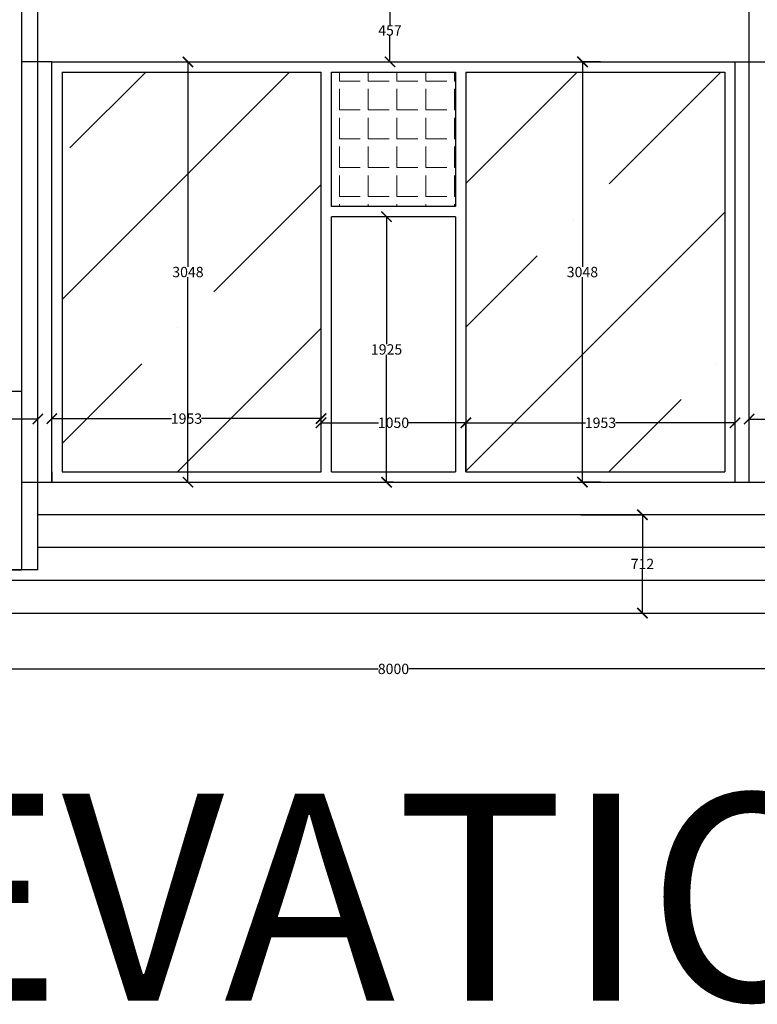
# Model space of a CAD drawing. Units: inches. Extents: x 829 to 33356404, y 1874 to 16983.
# Tile 6 of 9: x 10848 to 16199, y 1874 to 9014. Entities that reach past the tile are written whole.
import ezdxf

# ---------------------------------------------------------------- set-up
doc = ezdxf.new("R2010")
doc.units = ezdxf.units.IN
doc.header["$MEASUREMENT"] = 0
doc.header["$PDMODE"] = 3
for name, color, linetype, lineweight in [('A-ANNO-DIMS', 2, 'Continuous', 18), ('A-ANNO-TEXT', 7, 'Continuous', 25), ('A-ELEV', 7, 'Continuous', 25), ('A-ELEV-PATT', 8, 'Continuous', 13)]:
    doc.layers.add(name, color=color, linetype=linetype, lineweight=lineweight)
doc.styles.get("Standard").update_dxf_attribs({"font": 'arial.ttf'})
doc.dimstyles.get("Standard").update_dxf_attribs({"dimtxt": 75, "dimasz": 75, "dimexe": 0.18, "dimexo": 0.0625, "dimgap": 0.09, "dimtad": 0, "dimtih": 1, "dimtoh": 1, "dimdec": 0, "dimzin": 0, "dimdsep": 46, "dimtxsty": 'Standard', "dimblk": 'ARCHTICK', "dimcen": 0.09, "dimadec": 0, "dimazin": 0, "dimtfac": 1, "dimtdec": 0, "dimtofl": 0, "dimtmove": 0, "dimatfit": 3, "dimfxl": 1, "dimtolj": 1, "dimtzin": 0, "dimarcsym": 0})

# ---------------------------------------------------------------- blocks, each defined once
blk = doc.blocks.new('_ArchTick')
at = {"color": 0, "linetype": 'ByBlock', "const_width": 0.15}
blk.add_lwpolyline([(-0.5, -0.5), (0.5, 0.5)], dxfattribs=at)
blk = doc.blocks.new('*D3')
at = {"layer": 'A-ANNO-DIMS', "color": 0, "lineweight": -2, "transparency": 16777216}
for p, q in [((9559.8, 4746.4), (9559.8, 4306.1)), ((17559.8, 4746.4), (17559.8, 4306.1)), ((9559.8, 4306.3), (13447.8, 4306.3)), ((17559.8, 4306.3), (13671.8, 4306.3))]:
    blk.add_line(p, q, dxfattribs=at)
at = {"layer": 'Defpoints', "color": 0, "transparency": 16777216}
for p in [(9559.8, 4746.5), (17559.8, 4746.5), (17559.8, 4306.3)]:
    blk.add_point(p, dxfattribs=at)
at = {"layer": 'A-ANNO-DIMS', "color": 0, "lineweight": -2, "transparency": 16777216, "xscale": 75, "yscale": 75, "zscale": 75, "rotation": 180}
blk.add_blockref('_ArchTick', (9559.8, 4306.3), dxfattribs=at)
at = {"layer": 'A-ANNO-DIMS', "color": 0, "lineweight": -2, "transparency": 16777216, "xscale": 75, "yscale": 75, "zscale": 75}
blk.add_blockref('_ArchTick', (17559.8, 4306.3), dxfattribs=at)
at = {"layer": 'A-ANNO-DIMS', "color": 0, "transparency": 16777216, "insert": (13559.8, 4306.3), "char_height": 75, "attachment_point": 5}
blk.add_mtext('\\A1;8000', dxfattribs=at)
blk = doc.blocks.new('*D17')
at = {"layer": 'A-ANNO-DIMS', "color": 0, "lineweight": -2, "transparency": 16777216}
for p, q in [((9559.8, 5735.5), (9559.8, 6118.2)), ((9559.8, 6118), (10161.4, 6118)), ((10979.9, 6118), (10378.3, 6118)), ((10979.9, 5735.5), (10979.9, 6118.2))]:
    blk.add_line(p, q, dxfattribs=at)
at = {"layer": 'Defpoints', "color": 0, "transparency": 16777216}
for p in [(9559.8, 6118), (9559.8, 5735.5), (10979.9, 5735.5)]:
    blk.add_point(p, dxfattribs=at)
at = {"layer": 'A-ANNO-DIMS', "color": 0, "lineweight": -2, "transparency": 16777216, "xscale": 75, "yscale": 75, "zscale": 75, "rotation": 180}
blk.add_blockref('_ArchTick', (9559.8, 6118), dxfattribs=at)
at = {"layer": 'A-ANNO-DIMS', "color": 0, "lineweight": -2, "transparency": 16777216, "xscale": 75, "yscale": 75, "zscale": 75}
blk.add_blockref('_ArchTick', (10979.9, 6118), dxfattribs=at)
at = {"layer": 'A-ANNO-DIMS', "color": 0, "transparency": 16777216, "insert": (10269.9, 6118), "char_height": 75, "attachment_point": 5}
blk.add_mtext('\\A1;1420', dxfattribs=at)
blk = doc.blocks.new('*D18')
at = {"layer": 'A-ANNO-DIMS', "color": 0, "lineweight": -2, "transparency": 16777216}
for p, q in [((16139.7, 5735.5), (16139.7, 6118.2)), ((16139.7, 6118), (16741.3, 6118)), ((17559.8, 6118), (16958.2, 6118)), ((17559.8, 5735.5), (17559.8, 6118.2))]:
    blk.add_line(p, q, dxfattribs=at)
at = {"layer": 'Defpoints', "color": 0, "transparency": 16777216}
for p in [(16139.7, 6118), (16139.7, 5735.5), (17559.8, 5735.5)]:
    blk.add_point(p, dxfattribs=at)
at = {"layer": 'A-ANNO-DIMS', "color": 0, "lineweight": -2, "transparency": 16777216, "xscale": 75, "yscale": 75, "zscale": 75, "rotation": 180}
blk.add_blockref('_ArchTick', (16139.7, 6118), dxfattribs=at)
at = {"layer": 'A-ANNO-DIMS', "color": 0, "lineweight": -2, "transparency": 16777216, "xscale": 75, "yscale": 75, "zscale": 75}
blk.add_blockref('_ArchTick', (17559.8, 6118), dxfattribs=at)
at = {"layer": 'A-ANNO-DIMS', "color": 0, "transparency": 16777216, "insert": (16849.7, 6118), "char_height": 75, "attachment_point": 5}
blk.add_mtext('\\A1;1420', dxfattribs=at)
blk = doc.blocks.new('*D19')
at = {"layer": 'A-ANNO-DIMS', "color": 0, "lineweight": -2, "transparency": 16777216}
for p, q in [((14084.8, 5735.5), (14084.8, 6091.3)), ((14084.8, 6091.1), (14952.7, 6091.1)), ((16037.8, 6091.1), (15169.8, 6091.1)), ((16037.8, 5735.5), (16037.8, 6091.3))]:
    blk.add_line(p, q, dxfattribs=at)
at = {"layer": 'Defpoints', "color": 0, "transparency": 16777216}
for p in [(16037.8, 6091.1), (14084.8, 5735.5), (16037.8, 5735.5)]:
    blk.add_point(p, dxfattribs=at)
at = {"layer": 'A-ANNO-DIMS', "color": 0, "lineweight": -2, "transparency": 16777216, "xscale": 75, "yscale": 75, "zscale": 75, "rotation": 180}
blk.add_blockref('_ArchTick', (14084.8, 6091.1), dxfattribs=at)
at = {"layer": 'A-ANNO-DIMS', "color": 0, "lineweight": -2, "transparency": 16777216, "xscale": 75, "yscale": 75, "zscale": 75}
blk.add_blockref('_ArchTick', (16037.8, 6091.1), dxfattribs=at)
at = {"layer": 'A-ANNO-DIMS', "color": 0, "transparency": 16777216, "insert": (15061.3, 6091.1), "char_height": 75, "attachment_point": 5}
blk.add_mtext('\\A1;1953', dxfattribs=at)
blk = doc.blocks.new('*D20')
at = {"layer": 'A-ANNO-DIMS', "color": 0, "lineweight": -2, "transparency": 16777216}
for p, q in [((11081.8, 5735.5), (11081.8, 6121.5)), ((11081.8, 6121.3), (11949.7, 6121.3)), ((13034.8, 6121.3), (12166.8, 6121.3)), ((13034.8, 5735.5), (13034.8, 6121.5))]:
    blk.add_line(p, q, dxfattribs=at)
at = {"layer": 'Defpoints', "color": 0, "transparency": 16777216}
for p in [(13034.8, 6121.3), (11081.8, 5735.5), (13034.8, 5735.5)]:
    blk.add_point(p, dxfattribs=at)
at = {"layer": 'A-ANNO-DIMS', "color": 0, "lineweight": -2, "transparency": 16777216, "xscale": 75, "yscale": 75, "zscale": 75, "rotation": 180}
blk.add_blockref('_ArchTick', (11081.8, 6121.3), dxfattribs=at)
at = {"layer": 'A-ANNO-DIMS', "color": 0, "lineweight": -2, "transparency": 16777216, "xscale": 75, "yscale": 75, "zscale": 75}
blk.add_blockref('_ArchTick', (13034.8, 6121.3), dxfattribs=at)
at = {"layer": 'A-ANNO-DIMS', "color": 0, "transparency": 16777216, "insert": (12058.3, 6121.3), "char_height": 75, "attachment_point": 5}
blk.add_mtext('\\A1;1953', dxfattribs=at)
blk = doc.blocks.new('*D21')
at = {"layer": 'A-ANNO-DIMS', "color": 0, "lineweight": -2, "transparency": 16777216}
for p, q in [((15061.2, 8708.5), (14930.7, 8708.5)), ((14930.8, 8708.5), (14930.8, 7222.9)), ((14930.8, 5660.5), (14930.8, 7146.1)), ((15061.2, 5660.5), (14930.7, 5660.5))]:
    blk.add_line(p, q, dxfattribs=at)
at = {"layer": 'Defpoints', "color": 0, "transparency": 16777216}
for p in [(15061.3, 8708.5), (14930.8, 5660.5), (15061.3, 5660.5)]:
    blk.add_point(p, dxfattribs=at)
at = {"layer": 'A-ANNO-DIMS', "color": 0, "lineweight": -2, "transparency": 16777216, "xscale": 75, "yscale": 75, "zscale": 75}
for p, rotation in [((14930.8, 8708.5), 90), ((14930.8, 5660.5), 270)]:
    blk.add_blockref('_ArchTick', p, dxfattribs=dict(at, rotation=rotation))
at = {"layer": 'A-ANNO-DIMS', "color": 0, "transparency": 16777216, "insert": (14930.8, 7184.5), "char_height": 75, "attachment_point": 5}
blk.add_mtext('\\A1;3048', dxfattribs=at)
blk = doc.blocks.new('*D24')
at = {"layer": 'A-ANNO-DIMS', "color": 0, "lineweight": -2, "transparency": 16777216}
for p, q in [((13534.6, 9165.5), (13534.3, 9165.5)), ((13534.5, 9165.5), (13534.5, 8975.2)), ((13534.5, 8708.5), (13534.5, 8898.7)), ((13534.6, 8708.5), (13534.3, 8708.5))]:
    blk.add_line(p, q, dxfattribs=at)
at = {"layer": 'Defpoints', "color": 0, "transparency": 16777216}
for p in [(13534.7, 9165.5), (13534.5, 8708.5), (13534.7, 8708.5)]:
    blk.add_point(p, dxfattribs=at)
at = {"layer": 'A-ANNO-DIMS', "color": 0, "lineweight": -2, "transparency": 16777216, "xscale": 75, "yscale": 75, "zscale": 75}
for p, rotation in [((13534.5, 9165.5), 90), ((13534.5, 8708.5), 270)]:
    blk.add_blockref('_ArchTick', p, dxfattribs=dict(at, rotation=rotation))
at = {"layer": 'A-ANNO-DIMS', "color": 0, "transparency": 16777216, "insert": (13534.5, 8937), "char_height": 75, "attachment_point": 5}
blk.add_mtext('\\A1;457', dxfattribs=at)
blk = doc.blocks.new('*D34')
at = {"layer": 'A-ANNO-DIMS', "color": 0, "lineweight": -2, "transparency": 16777216}
for p, q in [((9559.8, 5735.5), (9559.8, 6118.2)), ((9559.8, 6118), (10161.4, 6118)), ((10979.9, 6118), (10378.2, 6118)), ((10979.9, 5735.5), (10979.9, 6118.2))]:
    blk.add_line(p, q, dxfattribs=at)
at = {"layer": 'Defpoints', "color": 0, "transparency": 16777216}
for p in [(10979.9, 6118), (9559.8, 5735.5), (10979.9, 5735.5)]:
    blk.add_point(p, dxfattribs=at)
at = {"layer": 'A-ANNO-DIMS', "color": 0, "lineweight": -2, "transparency": 16777216, "xscale": 75, "yscale": 75, "zscale": 75, "rotation": 180}
blk.add_blockref('_ArchTick', (9559.8, 6118), dxfattribs=at)
at = {"layer": 'A-ANNO-DIMS', "color": 0, "lineweight": -2, "transparency": 16777216, "xscale": 75, "yscale": 75, "zscale": 75}
blk.add_blockref('_ArchTick', (10979.9, 6118), dxfattribs=at)
at = {"layer": 'A-ANNO-DIMS', "color": 0, "transparency": 16777216, "insert": (10269.8, 6118), "char_height": 75, "attachment_point": 5}
blk.add_mtext('\\A1;1420', dxfattribs=at)
blk = doc.blocks.new('*D60')
at = {"layer": 'A-ANNO-DIMS', "color": 0, "lineweight": -2, "transparency": 16777216}
for p, q in [((14918.4, 5423.5), (15365.9, 5423.5)), ((15365.7, 5423.5), (15365.7, 5105.2)), ((15365.7, 4711.5), (15365.7, 5029.8)), ((14972.8, 4711.5), (15365.9, 4711.5))]:
    blk.add_line(p, q, dxfattribs=at)
at = {"layer": 'Defpoints', "color": 0, "transparency": 16777216}
for p in [(14918.4, 5423.5), (14972.7, 4711.5), (15365.7, 4711.5)]:
    blk.add_point(p, dxfattribs=at)
at = {"layer": 'A-ANNO-DIMS', "color": 0, "lineweight": -2, "transparency": 16777216, "xscale": 75, "yscale": 75, "zscale": 75}
for p, rotation in [((15365.7, 5423.5), 90), ((15365.7, 4711.5), 270)]:
    blk.add_blockref('_ArchTick', p, dxfattribs=dict(at, rotation=rotation))
at = {"layer": 'A-ANNO-DIMS', "color": 0, "transparency": 16777216, "insert": (15365.7, 5067.5), "char_height": 75, "attachment_point": 5}
blk.add_mtext('\\A1;712', dxfattribs=at)
blk = doc.blocks.new('*D61')
at = {"layer": 'A-ANNO-DIMS', "color": 0, "lineweight": -2, "transparency": 16777216}
for p, q in [((12058.3, 8708.5), (12069.1, 8708.5)), ((12068.9, 8708.5), (12068.9, 7222.9)), ((12068.9, 5660.5), (12068.9, 7146.1)), ((12058.3, 5660.5), (12069.1, 5660.5))]:
    blk.add_line(p, q, dxfattribs=at)
at = {"layer": 'Defpoints', "color": 0, "transparency": 16777216}
for p in [(12058.3, 8708.5), (12058.3, 5660.5), (12068.9, 5660.5)]:
    blk.add_point(p, dxfattribs=at)
at = {"layer": 'A-ANNO-DIMS', "color": 0, "lineweight": -2, "transparency": 16777216, "xscale": 75, "yscale": 75, "zscale": 75}
for p, rotation in [((12068.9, 8708.5), 90), ((12068.9, 5660.5), 270)]:
    blk.add_blockref('_ArchTick', p, dxfattribs=dict(at, rotation=rotation))
at = {"layer": 'A-ANNO-DIMS', "color": 0, "transparency": 16777216, "insert": (12068.9, 7184.5), "char_height": 75, "attachment_point": 5}
blk.add_mtext('\\A1;3048', dxfattribs=at)
blk = doc.blocks.new('*D62')
at = {"layer": 'A-ANNO-DIMS', "color": 0, "lineweight": -2, "transparency": 16777216}
for p, q in [((13559.7, 7585.5), (13509.7, 7585.5)), ((13509.8, 7585.5), (13509.8, 6661.4)), ((13509.8, 5660.5), (13509.8, 6584.6)), ((13559.7, 5660.5), (13509.7, 5660.5))]:
    blk.add_line(p, q, dxfattribs=at)
at = {"layer": 'Defpoints', "color": 0, "transparency": 16777216}
for p in [(13509.8, 7585.5), (13559.8, 7585.5), (13559.8, 5660.5)]:
    blk.add_point(p, dxfattribs=at)
at = {"layer": 'A-ANNO-DIMS', "color": 0, "lineweight": -2, "transparency": 16777216, "xscale": 75, "yscale": 75, "zscale": 75}
for p, rotation in [((13509.8, 7585.5), 90), ((13509.8, 5660.5), 270)]:
    blk.add_blockref('_ArchTick', p, dxfattribs=dict(at, rotation=rotation))
at = {"layer": 'A-ANNO-DIMS', "color": 0, "transparency": 16777216, "insert": (13509.8, 6623), "char_height": 75, "attachment_point": 5}
blk.add_mtext('\\A1;1925', dxfattribs=at)
blk = doc.blocks.new('*D63')
at = {"layer": 'A-ANNO-DIMS', "color": 0, "lineweight": -2, "transparency": 16777216}
for p, q in [((13034.8, 5735.5), (13034.8, 6091.4)), ((13034.8, 6091.3), (13451.4, 6091.3)), ((14084.8, 6091.3), (13668.2, 6091.3)), ((14084.8, 6091.3), (14084.8, 6091.4))]:
    blk.add_line(p, q, dxfattribs=at)
at = {"layer": 'Defpoints', "color": 0, "transparency": 16777216}
for p in [(14084.8, 6091.3), (14084.8, 6091.3), (13034.8, 5735.5)]:
    blk.add_point(p, dxfattribs=at)
at = {"layer": 'A-ANNO-DIMS', "color": 0, "lineweight": -2, "transparency": 16777216, "xscale": 75, "yscale": 75, "zscale": 75, "rotation": 180}
blk.add_blockref('_ArchTick', (13034.8, 6091.3), dxfattribs=at)
at = {"layer": 'A-ANNO-DIMS', "color": 0, "lineweight": -2, "transparency": 16777216, "xscale": 75, "yscale": 75, "zscale": 75}
blk.add_blockref('_ArchTick', (14084.8, 6091.3), dxfattribs=at)
at = {"layer": 'A-ANNO-DIMS', "color": 0, "transparency": 16777216, "insert": (13559.8, 6091.3), "char_height": 75, "attachment_point": 5}
blk.add_mtext('\\A1;1050', dxfattribs=at)
blk = doc.blocks.new('*D83')
at = {"layer": 'A-ANNO-DIMS', "color": 0, "lineweight": -2, "transparency": 16777216}
for p, q in [((13604.5, 15734.9), (985.4, 15734.9)), ((985.6, 15734.9), (985.6, 10279.1)), ((985.6, 4746.5), (985.6, 10202.3)), ((3169.7, 4746.5), (985.4, 4746.5))]:
    blk.add_line(p, q, dxfattribs=at)
at = {"layer": 'Defpoints', "color": 0, "transparency": 16777216}
for p in [(985.6, 15734.9), (13604.5, 15734.9), (3169.8, 4746.5)]:
    blk.add_point(p, dxfattribs=at)
at = {"layer": 'A-ANNO-DIMS', "color": 0, "lineweight": -2, "transparency": 16777216, "xscale": 75, "yscale": 75, "zscale": 75}
for p, rotation in [((985.6, 15734.9), 90), ((985.6, 4746.5), 270)]:
    blk.add_blockref('_ArchTick', p, dxfattribs=dict(at, rotation=rotation))
at = {"layer": 'A-ANNO-DIMS', "color": 0, "transparency": 16777216, "insert": (985.6, 10240.7), "char_height": 75, "attachment_point": 5}
blk.add_mtext('\\A1;10988', dxfattribs=at)
blk = doc.blocks.new('*D91')
at = {"layer": 'A-ANNO-DIMS', "color": 0, "lineweight": -2, "transparency": 16777216}
for p, q in [((11081.8, 9925.5), (26134.1, 9925.5)), ((26133.9, 9925.5), (26133.9, 9354.7)), ((26133.9, 8708.5), (26133.9, 9279.2)), ((11081.8, 8708.5), (26134.1, 8708.5))]:
    blk.add_line(p, q, dxfattribs=at)
at = {"layer": 'Defpoints', "color": 0, "transparency": 16777216}
for p in [(11081.8, 9925.5), (11081.8, 8708.5), (26133.9, 8708.5)]:
    blk.add_point(p, dxfattribs=at)
at = {"layer": 'A-ANNO-DIMS', "color": 0, "lineweight": -2, "transparency": 16777216, "xscale": 75, "yscale": 75, "zscale": 75}
for p, rotation in [((26133.9, 9925.5), 90), ((26133.9, 8708.5), 270)]:
    blk.add_blockref('_ArchTick', p, dxfattribs=dict(at, rotation=rotation))
at = {"layer": 'A-ANNO-DIMS', "color": 0, "transparency": 16777216, "insert": (26133.9, 9317), "char_height": 75, "attachment_point": 5}
blk.add_mtext('\\A1;1217', dxfattribs=at)

msp = doc.modelspace()

# ---------------------------------------------------------------- hatches: boundary and pattern name
at = {"layer": 'A-ELEV-PATT'}
h = msp.add_hatch(dxfattribs=at)
h.set_pattern_fill('ANSI35', color=256, scale=5900)
h.paths.add_polyline_path([(11156.778, 8633.468), (11156.778, 5735.468), (13034.778, 5735.468), (13034.778, 8633.468)])
h = msp.add_hatch(dxfattribs=at)
h.set_pattern_fill('ANGLE', color=256, scale=760)
h.set_pattern_definition([(0, (0, 0), (0, 209), [152, -57]), (90, (0, 0), (-209, 1e-14), [152, -57])])
h.paths.add_polyline_path([(14009.778, 8633.468), (13109.778, 8633.468), (13109.778, 7660.468), (14009.778, 7660.468)])
h = msp.add_hatch(dxfattribs=at)
h.set_pattern_fill('ANSI35', color=256, scale=5900)
h.paths.add_polyline_path([(15962.778, 8633.468), (14084.778, 8633.468), (14084.778, 5735.468), (15962.778, 5735.468)])
h.paths.add_polyline_path([(14922.661, 6013.301), (15193.244, 6013.301), (15193.244, 6167.854), (14922.661, 6167.854)], flags=24)
h.paths.add_polyline_path([(14795.645, 7106.68), (15066.228, 7106.68), (15066.228, 7261.233), (14795.645, 7261.233)], flags=24)

# ---------------------------------------------------------------- linework, layer by layer
at = {"layer": 'A-ELEV'}
for p, q in [((10860.89, 12127.212), (10860.89, 5024.468)), ((10979.778, 5024.468), (10979.778, 12127.212)), ((16139.778, 5660.468), (16139.778, 12127.212)), ((11081.778, 8708.468), (10860.89, 8708.468)), ((11081.778, 5660.468), (11081.778, 8708.468)), ((11081.778, 8708.468), (13034.778, 8708.468)), ((14084.778, 8708.468), (16037.778, 8708.468)), ((16037.778, 5660.468), (16037.778, 8708.468)), ((11156.778, 8633.468), (13034.778, 8633.468)), ((11156.778, 8633.468), (11156.778, 5735.468)), ((14084.778, 8633.468), (15962.778, 8633.468)), ((15962.778, 8633.468), (15962.778, 5735.468)), ((14009.778, 7660.468), (13109.778, 7660.468)), ((14009.778, 7585.468), (13109.778, 7585.468)), ((9559.807, 6321.468), (10860.89, 6321.304)), ((11081.778, 5735.468), (11081.778, 5660.468)), ((11156.778, 5735.468), (13034.778, 5735.468)), ((13109.778, 5735.468), (14009.778, 5735.468)), ((14084.778, 5735.468), (15962.778, 5735.468)), ((10860.89, 5660.468), (16258.701, 5660.468)), ((16258.701, 5423.468), (10979.778, 5423.468)), ((16258.701, 5186.468), (10979.778, 5186.468)), ((9559.692, 5024.468), (10860.89, 5024.468)), ((10979.778, 5024.468), (9559.778, 5024.468)), ((9559.778, 4949.468), (17559.778, 4949.468)), ((9559.778, 4711.528), (17559.778, 4711.528))]:
    msp.add_line(p, q, dxfattribs=at)
for points in [[(13034.778, 8708.468), (14084.778, 8708.468)], [(13034.778, 5735.468), (13034.778, 8633.468)], [(13109.778, 7660.468), (13109.778, 8633.468), (14009.778, 8633.468), (14009.778, 7660.468)], [(14084.778, 8633.468), (14084.778, 5735.468)], [(13109.778, 5735.468), (13109.778, 7585.468)], [(14009.778, 7585.468), (14009.778, 5735.468)]]:
    msp.add_lwpolyline(points, dxfattribs=at)

# ---------------------------------------------------------------- texts
at = {"layer": 'A-ANNO-TEXT'}
msp.add_text('ELEVATION', height=1500, dxfattribs=at).set_placement((7631.721, 1900.346))

# ---------------------------------------------------------------- dimensions: what is measured, and where the dimension line sits
at = {"layer": 'A-ANNO-DIMS'}
for base, p1, p2, angle, override, picture, middle in [((985.628, 15734.879), (3169.778, 4746.468), (13604.527, 15734.879), 90, {"dimdec": 0, "dimlfac": 1, "dimrnd": 0, "dimzin": 0, "dimdsep": 46, "dimlunit": 2}, '*D83', (985.628, 10240.673)), ((26133.929, 8708.468), (11081.778, 9925.468), (11081.778, 8708.468), 90, {"dimdec": 0, "dimlfac": 1, "dimrnd": 0, "dimzin": 0, "dimdsep": 46, "dimlunit": 2}, '*D91', (26133.929, 9316.968)), ((13534.477, 8708.468), (13534.687, 9165.468), (13534.687, 8708.468), 90, {"dimclrd": 0, "dimclre": 0, "dimclrt": 0}, '*D24', (13534.477, 8936.968)), ((12068.89, 5660.468), (12058.278, 8708.468), (12058.278, 5660.468), 90, {"dimclrd": 0, "dimclre": 0, "dimclrt": 0}, '*D61', (12068.89, 7184.468)), ((14930.834, 5660.468), (15061.278, 8708.468), (15061.278, 5660.468), 90, {"dimclrd": 0, "dimclre": 0, "dimclrt": 0}, '*D21', (14930.834, 7184.468)), ((13509.831, 7585.468), (13559.796, 5660.468), (13559.796, 7585.468), 90, {"dimclrd": 0, "dimclre": 0, "dimclrt": 0}, '*D62', (13509.831, 6622.968)), ((10979.871, 6118.028), (9559.778, 5735.468), (10979.871, 5735.461), 180, {"dimclrd": 0, "dimclre": 0, "dimclrt": 0}, '*D34', (10269.825, 6118.028)), ((15365.741, 4711.528), (14918.359, 5423.468), (14972.743, 4711.528), 90, {"dimclrd": 0, "dimclre": 0, "dimclrt": 0}, '*D60', (15365.741, 5067.498))]:
    dim = msp.add_linear_dim(base=base, p1=p1, p2=p2, angle=angle, dimstyle='Standard', override=override, dxfattribs=at)
    dim.commit()
    dim.dimension.update_dxf_attribs({"geometry": picture, "text_midpoint": middle})
for base, p1, p2, picture, middle in [((9559.81, 6118.028), (10979.903, 5735.468), (9559.81, 5735.461), '*D17', (10269.856, 6118.028)), ((13034.778, 6121.293), (11081.778, 5735.468), (13034.778, 5735.468), '*D20', (12058.278, 6121.293)), ((16139.685, 6118.028), (17559.778, 5735.468), (16139.685, 5735.461), '*D18', (16849.732, 6118.028)), ((14084.778, 6091.269), (13034.778, 5735.468), (14084.778, 6091.269), '*D63', (13559.778, 6091.269)), ((16037.778, 6091.089), (14084.778, 5735.468), (16037.778, 5735.468), '*D19', (15061.278, 6091.089)), ((17559.778, 4306.306), (9559.778, 4746.468), (17559.778, 4746.468), '*D3', (13559.778, 4306.306))]:
    dim = msp.add_linear_dim(base=base, p1=p1, p2=p2, dimstyle='Standard', override={"dimclrd": 0, "dimclre": 0, "dimclrt": 0}, dxfattribs=at)
    dim.commit()
    dim.dimension.update_dxf_attribs({"geometry": picture, "text_midpoint": middle})

doc.saveas('drawing.dxf')
